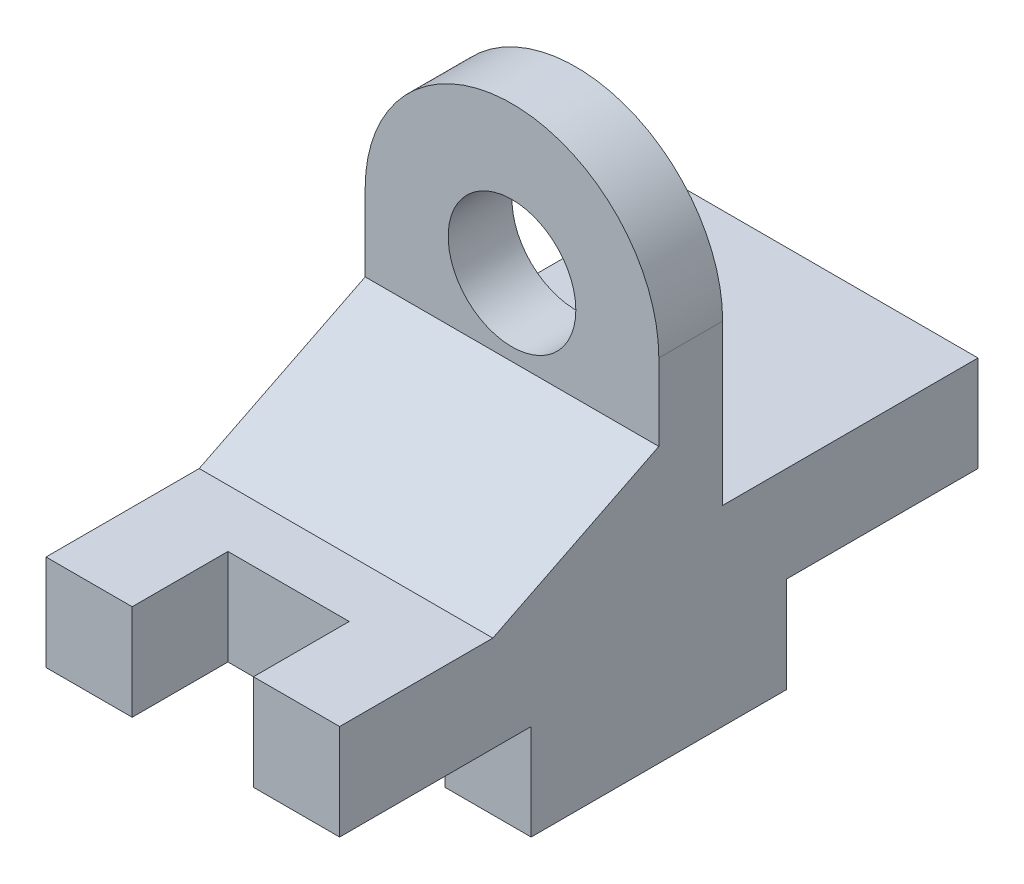
ISO-10303-21;
HEADER;
FILE_DESCRIPTION(('STEP AP214'),'2;1');
FILE_NAME('part.step','',(''),(''),'','','');
FILE_SCHEMA(('AUTOMOTIVE_DESIGN { 1 0 10303 214 1 1 1 1 }'));
ENDSEC;
DATA;
#1=APPLICATION_CONTEXT('core data for automotive mechanical design processes');
#2=APPLICATION_PROTOCOL_DEFINITION('international standard','automotive_design',2000,#1);
#3=PRODUCT_CONTEXT('',#1,'mechanical');
#4=PRODUCT('Part','Part','',(#3));
#5=PRODUCT_RELATED_PRODUCT_CATEGORY('part','',(#4));
#6=PRODUCT_DEFINITION_FORMATION('','',#4);
#7=PRODUCT_DEFINITION_CONTEXT('part definition',#1,'design');
#8=PRODUCT_DEFINITION('design','',#6,#7);
#9=PRODUCT_DEFINITION_SHAPE('','',#8);
#10=(LENGTH_UNIT() NAMED_UNIT(*) SI_UNIT(.MILLI.,.METRE.));
#11=(NAMED_UNIT(*) PLANE_ANGLE_UNIT() SI_UNIT($,.RADIAN.));
#12=(NAMED_UNIT(*) SI_UNIT($,.STERADIAN.) SOLID_ANGLE_UNIT());
#13=UNCERTAINTY_MEASURE_WITH_UNIT(LENGTH_MEASURE(1.E-05),#10,'distance_accuracy_value','');
#14=(GEOMETRIC_REPRESENTATION_CONTEXT(3) GLOBAL_UNCERTAINTY_ASSIGNED_CONTEXT((#13)) GLOBAL_UNIT_ASSIGNED_CONTEXT((#10,
#11,#12)) REPRESENTATION_CONTEXT('',''));
#15=CARTESIAN_POINT('',(0.,0.,0.));
#16=DIRECTION('',(0.,0.,1.));
#17=DIRECTION('',(1.,0.,0.));
#18=AXIS2_PLACEMENT_3D('',#15,#16,#17);
#19=CARTESIAN_POINT('',(23.,0.,60.));
#20=DIRECTION('',(0.,-1.,0.));
#21=DIRECTION('',(0.,0.,-1.));
#22=AXIS2_PLACEMENT_3D('',#19,#20,#21);
#23=PLANE('',#22);
#24=DIRECTION('',(0.,0.,1.));
#25=VECTOR('',#24,1.);
#26=CARTESIAN_POINT('',(23.,0.,60.));
#27=LINE('',#26,#25);
#28=CARTESIAN_POINT('',(23.,0.,35.9999999999999));
#29=VERTEX_POINT('',#28);
#30=CARTESIAN_POINT('',(23.,0.,60.));
#31=VERTEX_POINT('',#30);
#32=EDGE_CURVE('E67',#29,#31,#27,.T.);
#33=ORIENTED_EDGE('',*,*,#32,.F.);
#34=DIRECTION('',(-1.,0.,0.));
#35=VECTOR('',#34,1.);
#36=CARTESIAN_POINT('',(23.,0.,36.));
#37=LINE('',#36,#35);
#38=CARTESIAN_POINT('',(-23.,0.,35.9999999999999));
#39=VERTEX_POINT('',#38);
#40=EDGE_CURVE('E71',#29,#39,#37,.T.);
#41=ORIENTED_EDGE('',*,*,#40,.T.);
#42=DIRECTION('',(0.,0.,1.));
#43=VECTOR('',#42,1.);
#44=CARTESIAN_POINT('',(-23.,0.,60.));
#45=LINE('',#44,#43);
#46=CARTESIAN_POINT('',(-23.,0.,60.));
#47=VERTEX_POINT('',#46);
#48=EDGE_CURVE('E314',#39,#47,#45,.T.);
#49=ORIENTED_EDGE('',*,*,#48,.T.);
#50=DIRECTION('',(-1.,0.,0.));
#51=VECTOR('',#50,1.);
#52=CARTESIAN_POINT('',(23.,0.,60.));
#53=LINE('',#52,#51);
#54=CARTESIAN_POINT('',(-9.5,0.,60.));
#55=VERTEX_POINT('',#54);
#56=EDGE_CURVE('E298',#55,#47,#53,.T.);
#57=ORIENTED_EDGE('',*,*,#56,.F.);
#58=DIRECTION('',(0.,0.,1.));
#59=VECTOR('',#58,1.);
#60=CARTESIAN_POINT('',(-9.5,0.,60.));
#61=LINE('',#60,#59);
#62=CARTESIAN_POINT('',(-9.5,0.,45.));
#63=VERTEX_POINT('',#62);
#64=EDGE_CURVE('E257',#63,#55,#61,.T.);
#65=ORIENTED_EDGE('',*,*,#64,.F.);
#66=DIRECTION('',(-1.,0.,0.));
#67=VECTOR('',#66,1.);
#68=CARTESIAN_POINT('',(-9.5,0.,45.));
#69=LINE('',#68,#67);
#70=CARTESIAN_POINT('',(9.5,0.,45.));
#71=VERTEX_POINT('',#70);
#72=EDGE_CURVE('E266',#71,#63,#69,.T.);
#73=ORIENTED_EDGE('',*,*,#72,.F.);
#74=DIRECTION('',(0.,0.,-1.));
#75=VECTOR('',#74,1.);
#76=CARTESIAN_POINT('',(9.5,0.,60.));
#77=LINE('',#76,#75);
#78=CARTESIAN_POINT('',(9.5,0.,60.));
#79=VERTEX_POINT('',#78);
#80=EDGE_CURVE('E263',#79,#71,#77,.T.);
#81=ORIENTED_EDGE('',*,*,#80,.F.);
#82=EDGE_CURVE('E320',#31,#79,#53,.T.);
#83=ORIENTED_EDGE('',*,*,#82,.F.);
#84=EDGE_LOOP('',(#33,#41,#49,#57,#65,#73,#81,#83));
#85=FACE_BOUND('',#84,.T.);
#86=ADVANCED_FACE('F53',(#85),#23,.F.);
#87=CARTESIAN_POINT('',(23.,-15.,30.));
#88=DIRECTION('',(0.,0.,-1.));
#89=DIRECTION('',(0.,1.,0.));
#90=AXIS2_PLACEMENT_3D('',#87,#88,#89);
#91=PLANE('',#90);
#92=DIRECTION('',(0.,-1.,0.));
#93=VECTOR('',#92,1.);
#94=CARTESIAN_POINT('',(9.5,29.2831796509691,30.));
#95=LINE('',#94,#93);
#96=CARTESIAN_POINT('',(9.5,-15.,30.));
#97=VERTEX_POINT('',#96);
#98=CARTESIAN_POINT('',(9.5,-30.,30.));
#99=VERTEX_POINT('',#98);
#100=EDGE_CURVE('E236',#97,#99,#95,.T.);
#101=ORIENTED_EDGE('',*,*,#100,.T.);
#102=DIRECTION('',(-1.,0.,0.));
#103=VECTOR('',#102,1.);
#104=CARTESIAN_POINT('',(23.,-30.,30.));
#105=LINE('',#104,#103);
#106=CARTESIAN_POINT('',(23.,-30.,30.));
#107=VERTEX_POINT('',#106);
#108=EDGE_CURVE('E333',#107,#99,#105,.T.);
#109=ORIENTED_EDGE('',*,*,#108,.F.);
#110=DIRECTION('',(0.,-1.,0.));
#111=VECTOR('',#110,1.);
#112=CARTESIAN_POINT('',(23.,-15.,30.));
#113=LINE('',#112,#111);
#114=CARTESIAN_POINT('',(23.,-15.,30.));
#115=VERTEX_POINT('',#114);
#116=EDGE_CURVE('E281',#115,#107,#113,.T.);
#117=ORIENTED_EDGE('',*,*,#116,.F.);
#118=DIRECTION('',(-1.,0.,0.));
#119=VECTOR('',#118,1.);
#120=CARTESIAN_POINT('',(23.,-15.,30.));
#121=LINE('',#120,#119);
#122=EDGE_CURVE('E336',#115,#97,#121,.T.);
#123=ORIENTED_EDGE('',*,*,#122,.T.);
#124=EDGE_LOOP('',(#101,#109,#117,#123));
#125=FACE_BOUND('',#124,.T.);
#126=ADVANCED_FACE('F399',(#125),#91,.F.);
#127=CARTESIAN_POINT('',(23.,-30.,30.));
#128=DIRECTION('',(0.,1.,0.));
#129=DIRECTION('',(0.,0.,1.));
#130=AXIS2_PLACEMENT_3D('',#127,#128,#129);
#131=PLANE('',#130);
#132=DIRECTION('',(0.,0.,1.));
#133=VECTOR('',#132,1.);
#134=CARTESIAN_POINT('',(9.5,-30.,30.));
#135=LINE('',#134,#133);
#136=CARTESIAN_POINT('',(9.5,-30.,-10.));
#137=VERTEX_POINT('',#136);
#138=EDGE_CURVE('E232',#99,#137,#135,.F.);
#139=ORIENTED_EDGE('',*,*,#138,.T.);
#140=DIRECTION('',(-1.,0.,0.));
#141=VECTOR('',#140,1.);
#142=CARTESIAN_POINT('',(23.,-30.,-10.));
#143=LINE('',#142,#141);
#144=CARTESIAN_POINT('',(23.,-30.,-10.));
#145=VERTEX_POINT('',#144);
#146=EDGE_CURVE('E332',#145,#137,#143,.T.);
#147=ORIENTED_EDGE('',*,*,#146,.F.);
#148=DIRECTION('',(0.,0.,-1.));
#149=VECTOR('',#148,1.);
#150=CARTESIAN_POINT('',(23.,-30.,30.));
#151=LINE('',#150,#149);
#152=EDGE_CURVE('E282',#107,#145,#151,.T.);
#153=ORIENTED_EDGE('',*,*,#152,.F.);
#154=ORIENTED_EDGE('',*,*,#108,.T.);
#155=EDGE_LOOP('',(#139,#147,#153,#154));
#156=FACE_BOUND('',#155,.T.);
#157=ADVANCED_FACE('F400',(#156),#131,.F.);
#158=CARTESIAN_POINT('',(23.,-30.,-10.));
#159=DIRECTION('',(0.,0.,1.));
#160=DIRECTION('',(1.,0.,0.));
#161=AXIS2_PLACEMENT_3D('',#158,#159,#160);
#162=PLANE('',#161);
#163=DIRECTION('',(0.,-1.,0.));
#164=VECTOR('',#163,1.);
#165=CARTESIAN_POINT('',(9.5,29.2831796509691,-10.));
#166=LINE('',#165,#164);
#167=CARTESIAN_POINT('',(9.5,-15.,-10.));
#168=VERTEX_POINT('',#167);
#169=EDGE_CURVE('E240',#168,#137,#166,.T.);
#170=ORIENTED_EDGE('',*,*,#169,.F.);
#171=DIRECTION('',(-1.,0.,0.));
#172=VECTOR('',#171,1.);
#173=CARTESIAN_POINT('',(23.,-15.,-10.));
#174=LINE('',#173,#172);
#175=CARTESIAN_POINT('',(23.,-15.,-10.));
#176=VERTEX_POINT('',#175);
#177=EDGE_CURVE('E330',#176,#168,#174,.T.);
#178=ORIENTED_EDGE('',*,*,#177,.F.);
#179=DIRECTION('',(0.,1.,0.));
#180=VECTOR('',#179,1.);
#181=CARTESIAN_POINT('',(23.,-30.,-10.));
#182=LINE('',#181,#180);
#183=EDGE_CURVE('E290',#145,#176,#182,.T.);
#184=ORIENTED_EDGE('',*,*,#183,.F.);
#185=ORIENTED_EDGE('',*,*,#146,.T.);
#186=EDGE_LOOP('',(#170,#178,#184,#185));
#187=FACE_BOUND('',#186,.T.);
#188=ADVANCED_FACE('F395',(#187),#162,.F.);
#189=CARTESIAN_POINT('',(23.,0.,60.));
#190=DIRECTION('',(0.,0.,-1.));
#191=DIRECTION('',(-1.,0.,0.));
#192=AXIS2_PLACEMENT_3D('',#189,#190,#191);
#193=PLANE('',#192);
#194=ORIENTED_EDGE('',*,*,#82,.T.);
#195=DIRECTION('',(0.,1.,0.));
#196=VECTOR('',#195,1.);
#197=CARTESIAN_POINT('',(9.5,-30.001,60.));
#198=LINE('',#197,#196);
#199=CARTESIAN_POINT('',(9.5,-15.,60.));
#200=VERTEX_POINT('',#199);
#201=EDGE_CURVE('E274',#200,#79,#198,.T.);
#202=ORIENTED_EDGE('',*,*,#201,.F.);
#203=DIRECTION('',(-1.,0.,0.));
#204=VECTOR('',#203,1.);
#205=CARTESIAN_POINT('',(23.,-15.,60.));
#206=LINE('',#205,#204);
#207=CARTESIAN_POINT('',(23.,-15.,60.));
#208=VERTEX_POINT('',#207);
#209=EDGE_CURVE('E12',#208,#200,#206,.T.);
#210=ORIENTED_EDGE('',*,*,#209,.F.);
#211=DIRECTION('',(0.,-1.,0.));
#212=VECTOR('',#211,1.);
#213=CARTESIAN_POINT('',(23.,0.,60.));
#214=LINE('',#213,#212);
#215=EDGE_CURVE('E279',#31,#208,#214,.T.);
#216=ORIENTED_EDGE('',*,*,#215,.F.);
#217=EDGE_LOOP('',(#194,#202,#210,#216));
#218=FACE_BOUND('',#217,.T.);
#219=ADVANCED_FACE('F410',(#218),#193,.F.);
#220=CARTESIAN_POINT('',(-23.,0.,-40.));
#221=VERTEX_POINT('',#220);
#222=CARTESIAN_POINT('',(-23.,0.,0.));
#223=VERTEX_POINT('',#222);
#224=EDGE_CURVE('E283',#221,#223,#45,.T.);
#225=ORIENTED_EDGE('',*,*,#224,.T.);
#226=DIRECTION('',(1.,0.,0.));
#227=VECTOR('',#226,1.);
#228=CARTESIAN_POINT('',(-23.,0.,0.));
#229=LINE('',#228,#227);
#230=CARTESIAN_POINT('',(23.,0.,0.));
#231=VERTEX_POINT('',#230);
#232=EDGE_CURVE('E223',#223,#231,#229,.T.);
#233=ORIENTED_EDGE('',*,*,#232,.T.);
#234=CARTESIAN_POINT('',(23.,0.,-40.));
#235=VERTEX_POINT('',#234);
#236=EDGE_CURVE('E291',#235,#231,#27,.T.);
#237=ORIENTED_EDGE('',*,*,#236,.F.);
#238=DIRECTION('',(-1.,0.,0.));
#239=VECTOR('',#238,1.);
#240=CARTESIAN_POINT('',(23.,0.,-40.));
#241=LINE('',#240,#239);
#242=EDGE_CURVE('E319',#235,#221,#241,.T.);
#243=ORIENTED_EDGE('',*,*,#242,.T.);
#244=EDGE_LOOP('',(#225,#233,#237,#243));
#245=FACE_BOUND('',#244,.T.);
#246=ADVANCED_FACE('F377',(#245),#23,.F.);
#247=DIRECTION('',(0.,-1.,0.));
#248=VECTOR('',#247,1.);
#249=CARTESIAN_POINT('',(-23.,0.,60.));
#250=LINE('',#249,#248);
#251=CARTESIAN_POINT('',(-23.,-15.,60.));
#252=VERTEX_POINT('',#251);
#253=EDGE_CURVE('E275',#47,#252,#250,.T.);
#254=ORIENTED_EDGE('',*,*,#253,.T.);
#255=CARTESIAN_POINT('',(-9.5,-15.,60.));
#256=VERTEX_POINT('',#255);
#257=EDGE_CURVE('E65',#256,#252,#206,.T.);
#258=ORIENTED_EDGE('',*,*,#257,.F.);
#259=DIRECTION('',(0.,1.,0.));
#260=VECTOR('',#259,1.);
#261=CARTESIAN_POINT('',(-9.5,-30.001,60.));
#262=LINE('',#261,#260);
#263=EDGE_CURVE('E267',#256,#55,#262,.T.);
#264=ORIENTED_EDGE('',*,*,#263,.T.);
#265=ORIENTED_EDGE('',*,*,#56,.T.);
#266=EDGE_LOOP('',(#254,#258,#264,#265));
#267=FACE_BOUND('',#266,.T.);
#268=ADVANCED_FACE('F57',(#267),#193,.F.);
#269=CARTESIAN_POINT('',(-9.5,-30.,30.));
#270=VERTEX_POINT('',#269);
#271=CARTESIAN_POINT('',(-23.,-30.,30.));
#272=VERTEX_POINT('',#271);
#273=EDGE_CURVE('E331',#270,#272,#105,.T.);
#274=ORIENTED_EDGE('',*,*,#273,.F.);
#275=DIRECTION('',(0.,-1.,0.));
#276=VECTOR('',#275,1.);
#277=CARTESIAN_POINT('',(-9.5,29.2831796509691,30.));
#278=LINE('',#277,#276);
#279=CARTESIAN_POINT('',(-9.5,-15.,30.));
#280=VERTEX_POINT('',#279);
#281=EDGE_CURVE('E248',#280,#270,#278,.T.);
#282=ORIENTED_EDGE('',*,*,#281,.F.);
#283=CARTESIAN_POINT('',(-23.,-15.,30.));
#284=VERTEX_POINT('',#283);
#285=EDGE_CURVE('E340',#280,#284,#121,.T.);
#286=ORIENTED_EDGE('',*,*,#285,.T.);
#287=DIRECTION('',(0.,-1.,0.));
#288=VECTOR('',#287,1.);
#289=CARTESIAN_POINT('',(-23.,-15.,30.));
#290=LINE('',#289,#288);
#291=EDGE_CURVE('E303',#284,#272,#290,.T.);
#292=ORIENTED_EDGE('',*,*,#291,.T.);
#293=EDGE_LOOP('',(#274,#282,#286,#292));
#294=FACE_BOUND('',#293,.T.);
#295=ADVANCED_FACE('F346',(#294),#91,.F.);
#296=CARTESIAN_POINT('',(-9.5,-30.,-10.));
#297=VERTEX_POINT('',#296);
#298=CARTESIAN_POINT('',(-23.,-30.,-10.));
#299=VERTEX_POINT('',#298);
#300=EDGE_CURVE('E329',#297,#299,#143,.T.);
#301=ORIENTED_EDGE('',*,*,#300,.F.);
#302=DIRECTION('',(0.,0.,1.));
#303=VECTOR('',#302,1.);
#304=CARTESIAN_POINT('',(-9.5,-30.,30.));
#305=LINE('',#304,#303);
#306=EDGE_CURVE('E239',#270,#297,#305,.F.);
#307=ORIENTED_EDGE('',*,*,#306,.F.);
#308=ORIENTED_EDGE('',*,*,#273,.T.);
#309=DIRECTION('',(0.,0.,-1.));
#310=VECTOR('',#309,1.);
#311=CARTESIAN_POINT('',(-23.,-30.,30.));
#312=LINE('',#311,#310);
#313=EDGE_CURVE('E302',#272,#299,#312,.T.);
#314=ORIENTED_EDGE('',*,*,#313,.T.);
#315=EDGE_LOOP('',(#301,#307,#308,#314));
#316=FACE_BOUND('',#315,.T.);
#317=ADVANCED_FACE('F363',(#316),#131,.F.);
#318=CARTESIAN_POINT('',(-9.5,-15.,-10.));
#319=VERTEX_POINT('',#318);
#320=CARTESIAN_POINT('',(-23.,-15.,-10.));
#321=VERTEX_POINT('',#320);
#322=EDGE_CURVE('E326',#319,#321,#174,.T.);
#323=ORIENTED_EDGE('',*,*,#322,.F.);
#324=DIRECTION('',(0.,-1.,0.));
#325=VECTOR('',#324,1.);
#326=CARTESIAN_POINT('',(-9.5,29.2831796509691,-10.));
#327=LINE('',#326,#325);
#328=EDGE_CURVE('E242',#319,#297,#327,.T.);
#329=ORIENTED_EDGE('',*,*,#328,.T.);
#330=ORIENTED_EDGE('',*,*,#300,.T.);
#331=DIRECTION('',(0.,1.,0.));
#332=VECTOR('',#331,1.);
#333=CARTESIAN_POINT('',(-23.,-30.,-10.));
#334=LINE('',#333,#332);
#335=EDGE_CURVE('E307',#299,#321,#334,.T.);
#336=ORIENTED_EDGE('',*,*,#335,.T.);
#337=EDGE_LOOP('',(#323,#329,#330,#336));
#338=FACE_BOUND('',#337,.T.);
#339=ADVANCED_FACE('F366',(#338),#162,.F.);
#340=CARTESIAN_POINT('',(23.,-15.,-10.));
#341=DIRECTION('',(0.,1.,0.));
#342=DIRECTION('',(0.,0.,1.));
#343=AXIS2_PLACEMENT_3D('',#340,#341,#342);
#344=PLANE('',#343);
#345=DIRECTION('',(0.,0.,-1.));
#346=VECTOR('',#345,1.);
#347=CARTESIAN_POINT('',(-23.,-15.,-10.));
#348=LINE('',#347,#346);
#349=CARTESIAN_POINT('',(-23.,-15.,-40.));
#350=VERTEX_POINT('',#349);
#351=EDGE_CURVE('E309',#321,#350,#348,.T.);
#352=ORIENTED_EDGE('',*,*,#351,.T.);
#353=DIRECTION('',(-1.,0.,0.));
#354=VECTOR('',#353,1.);
#355=CARTESIAN_POINT('',(23.,-15.,-40.));
#356=LINE('',#355,#354);
#357=CARTESIAN_POINT('',(23.,-15.,-40.));
#358=VERTEX_POINT('',#357);
#359=EDGE_CURVE('E323',#358,#350,#356,.T.);
#360=ORIENTED_EDGE('',*,*,#359,.F.);
#361=DIRECTION('',(0.,0.,-1.));
#362=VECTOR('',#361,1.);
#363=CARTESIAN_POINT('',(23.,-15.,-10.));
#364=LINE('',#363,#362);
#365=EDGE_CURVE('E287',#176,#358,#364,.T.);
#366=ORIENTED_EDGE('',*,*,#365,.F.);
#367=ORIENTED_EDGE('',*,*,#177,.T.);
#368=DIRECTION('',(0.,0.,-1.));
#369=VECTOR('',#368,1.);
#370=CARTESIAN_POINT('',(9.5,-15.,30.));
#371=LINE('',#370,#369);
#372=EDGE_CURVE('E243',#97,#168,#371,.T.);
#373=ORIENTED_EDGE('',*,*,#372,.F.);
#374=ORIENTED_EDGE('',*,*,#122,.F.);
#375=DIRECTION('',(0.,0.,-1.));
#376=VECTOR('',#375,1.);
#377=CARTESIAN_POINT('',(23.,-15.,60.));
#378=LINE('',#377,#376);
#379=EDGE_CURVE('E278',#208,#115,#378,.T.);
#380=ORIENTED_EDGE('',*,*,#379,.F.);
#381=ORIENTED_EDGE('',*,*,#209,.T.);
#382=DIRECTION('',(0.,0.,1.));
#383=VECTOR('',#382,1.);
#384=CARTESIAN_POINT('',(9.5,-15.,60.));
#385=LINE('',#384,#383);
#386=CARTESIAN_POINT('',(9.5,-15.,45.));
#387=VERTEX_POINT('',#386);
#388=EDGE_CURVE('E241',#387,#200,#385,.T.);
#389=ORIENTED_EDGE('',*,*,#388,.F.);
#390=DIRECTION('',(1.,0.,0.));
#391=VECTOR('',#390,1.);
#392=CARTESIAN_POINT('',(-9.5,-15.,45.));
#393=LINE('',#392,#391);
#394=CARTESIAN_POINT('',(-9.5,-15.,45.));
#395=VERTEX_POINT('',#394);
#396=EDGE_CURVE('E255',#395,#387,#393,.T.);
#397=ORIENTED_EDGE('',*,*,#396,.F.);
#398=DIRECTION('',(0.,0.,-1.));
#399=VECTOR('',#398,1.);
#400=CARTESIAN_POINT('',(-9.5,-15.,60.));
#401=LINE('',#400,#399);
#402=EDGE_CURVE('E260',#256,#395,#401,.T.);
#403=ORIENTED_EDGE('',*,*,#402,.F.);
#404=ORIENTED_EDGE('',*,*,#257,.T.);
#405=DIRECTION('',(0.,0.,-1.));
#406=VECTOR('',#405,1.);
#407=CARTESIAN_POINT('',(-23.,-15.,60.));
#408=LINE('',#407,#406);
#409=EDGE_CURVE('E296',#252,#284,#408,.T.);
#410=ORIENTED_EDGE('',*,*,#409,.T.);
#411=ORIENTED_EDGE('',*,*,#285,.F.);
#412=DIRECTION('',(0.,0.,-1.));
#413=VECTOR('',#412,1.);
#414=CARTESIAN_POINT('',(-9.5,-15.,30.));
#415=LINE('',#414,#413);
#416=EDGE_CURVE('E235',#280,#319,#415,.T.);
#417=ORIENTED_EDGE('',*,*,#416,.T.);
#418=ORIENTED_EDGE('',*,*,#322,.T.);
#419=EDGE_LOOP('',(#352,#360,#366,#367,#373,#374,#380,#381,#389,#397,#403,#404,#410,#411,#417,#418));
#420=FACE_BOUND('',#419,.T.);
#421=ADVANCED_FACE('F351',(#420),#344,.F.);
#422=CARTESIAN_POINT('',(23.,-15.,-40.));
#423=DIRECTION('',(0.,0.,1.));
#424=DIRECTION('',(0.,-1.,0.));
#425=AXIS2_PLACEMENT_3D('',#422,#423,#424);
#426=PLANE('',#425);
#427=DIRECTION('',(0.,1.,0.));
#428=VECTOR('',#427,1.);
#429=CARTESIAN_POINT('',(-23.,-15.,-40.));
#430=LINE('',#429,#428);
#431=EDGE_CURVE('E315',#350,#221,#430,.T.);
#432=ORIENTED_EDGE('',*,*,#431,.T.);
#433=ORIENTED_EDGE('',*,*,#242,.F.);
#434=DIRECTION('',(0.,1.,0.));
#435=VECTOR('',#434,1.);
#436=CARTESIAN_POINT('',(23.,-15.,-40.));
#437=LINE('',#436,#435);
#438=EDGE_CURVE('E292',#358,#235,#437,.T.);
#439=ORIENTED_EDGE('',*,*,#438,.F.);
#440=ORIENTED_EDGE('',*,*,#359,.T.);
#441=EDGE_LOOP('',(#432,#433,#439,#440));
#442=FACE_BOUND('',#441,.T.);
#443=ADVANCED_FACE('F372',(#442),#426,.F.);
#444=CARTESIAN_POINT('',(23.,0.,0.));
#445=DIRECTION('',(1.,0.,0.));
#446=DIRECTION('',(0.,0.,-1.));
#447=AXIS2_PLACEMENT_3D('',#444,#445,#446);
#448=PLANE('',#447);
#449=DIRECTION('',(0.,-0.447213595499958,0.894427190999916));
#450=VECTOR('',#449,1.);
#451=CARTESIAN_POINT('',(23.,13.,10.));
#452=LINE('',#451,#450);
#453=CARTESIAN_POINT('',(23.,13.,10.));
#454=VERTEX_POINT('',#453);
#455=EDGE_CURVE('E424',#454,#29,#452,.T.);
#456=ORIENTED_EDGE('',*,*,#455,.T.);
#457=ORIENTED_EDGE('',*,*,#32,.T.);
#458=ORIENTED_EDGE('',*,*,#215,.T.);
#459=ORIENTED_EDGE('',*,*,#379,.T.);
#460=ORIENTED_EDGE('',*,*,#116,.T.);
#461=ORIENTED_EDGE('',*,*,#152,.T.);
#462=ORIENTED_EDGE('',*,*,#183,.T.);
#463=ORIENTED_EDGE('',*,*,#365,.T.);
#464=ORIENTED_EDGE('',*,*,#438,.T.);
#465=ORIENTED_EDGE('',*,*,#236,.T.);
#466=DIRECTION('',(0.,-1.,0.));
#467=VECTOR('',#466,1.);
#468=CARTESIAN_POINT('',(23.,25.,0.));
#469=LINE('',#468,#467);
#470=CARTESIAN_POINT('',(23.,25.,0.));
#471=VERTEX_POINT('',#470);
#472=EDGE_CURVE('E224',#471,#231,#469,.T.);
#473=ORIENTED_EDGE('',*,*,#472,.F.);
#474=DIRECTION('',(0.,0.,-1.));
#475=VECTOR('',#474,1.);
#476=CARTESIAN_POINT('',(23.,25.,10.));
#477=LINE('',#476,#475);
#478=CARTESIAN_POINT('',(23.,25.,10.));
#479=VERTEX_POINT('',#478);
#480=EDGE_CURVE('E213',#479,#471,#477,.T.);
#481=ORIENTED_EDGE('',*,*,#480,.F.);
#482=DIRECTION('',(0.,-1.,0.));
#483=VECTOR('',#482,1.);
#484=CARTESIAN_POINT('',(23.,25.,10.));
#485=LINE('',#484,#483);
#486=EDGE_CURVE('E201',#479,#454,#485,.T.);
#487=ORIENTED_EDGE('',*,*,#486,.T.);
#488=EDGE_LOOP('',(#456,#457,#458,#459,#460,#461,#462,#463,#464,#465,#473,#481,#487));
#489=FACE_BOUND('',#488,.T.);
#490=ADVANCED_FACE('F387',(#489),#448,.T.);
#491=CARTESIAN_POINT('',(-23.,0.,0.));
#492=DIRECTION('',(1.,0.,0.));
#493=DIRECTION('',(0.,0.,-1.));
#494=AXIS2_PLACEMENT_3D('',#491,#492,#493);
#495=PLANE('',#494);
#496=ORIENTED_EDGE('',*,*,#48,.F.);
#497=DIRECTION('',(0.,-0.447213595499958,0.894427190999916));
#498=VECTOR('',#497,1.);
#499=CARTESIAN_POINT('',(-23.,13.,10.));
#500=LINE('',#499,#498);
#501=CARTESIAN_POINT('',(-23.,13.,10.));
#502=VERTEX_POINT('',#501);
#503=EDGE_CURVE('E217',#502,#39,#500,.T.);
#504=ORIENTED_EDGE('',*,*,#503,.F.);
#505=DIRECTION('',(0.,-1.,0.));
#506=VECTOR('',#505,1.);
#507=CARTESIAN_POINT('',(-23.,25.,10.));
#508=LINE('',#507,#506);
#509=CARTESIAN_POINT('',(-23.,25.,10.));
#510=VERTEX_POINT('',#509);
#511=EDGE_CURVE('E199',#510,#502,#508,.T.);
#512=ORIENTED_EDGE('',*,*,#511,.F.);
#513=DIRECTION('',(0.,0.,-1.));
#514=VECTOR('',#513,1.);
#515=CARTESIAN_POINT('',(-23.,25.,10.));
#516=LINE('',#515,#514);
#517=CARTESIAN_POINT('',(-23.,25.,0.));
#518=VERTEX_POINT('',#517);
#519=EDGE_CURVE('E202',#510,#518,#516,.T.);
#520=ORIENTED_EDGE('',*,*,#519,.T.);
#521=DIRECTION('',(0.,-1.,0.));
#522=VECTOR('',#521,1.);
#523=CARTESIAN_POINT('',(-23.,25.,0.));
#524=LINE('',#523,#522);
#525=EDGE_CURVE('E229',#518,#223,#524,.T.);
#526=ORIENTED_EDGE('',*,*,#525,.T.);
#527=ORIENTED_EDGE('',*,*,#224,.F.);
#528=ORIENTED_EDGE('',*,*,#431,.F.);
#529=ORIENTED_EDGE('',*,*,#351,.F.);
#530=ORIENTED_EDGE('',*,*,#335,.F.);
#531=ORIENTED_EDGE('',*,*,#313,.F.);
#532=ORIENTED_EDGE('',*,*,#291,.F.);
#533=ORIENTED_EDGE('',*,*,#409,.F.);
#534=ORIENTED_EDGE('',*,*,#253,.F.);
#535=EDGE_LOOP('',(#496,#504,#512,#520,#526,#527,#528,#529,#530,#531,#532,#533,#534));
#536=FACE_BOUND('',#535,.T.);
#537=ADVANCED_FACE('F216',(#536),#495,.F.);
#538=CARTESIAN_POINT('',(-9.5,-30.001,60.));
#539=DIRECTION('',(-1.,0.,0.));
#540=DIRECTION('',(0.,0.,1.));
#541=AXIS2_PLACEMENT_3D('',#538,#539,#540);
#542=PLANE('',#541);
#543=ORIENTED_EDGE('',*,*,#64,.T.);
#544=ORIENTED_EDGE('',*,*,#263,.F.);
#545=ORIENTED_EDGE('',*,*,#402,.T.);
#546=DIRECTION('',(0.,1.,0.));
#547=VECTOR('',#546,1.);
#548=CARTESIAN_POINT('',(-9.5,-30.001,45.));
#549=LINE('',#548,#547);
#550=EDGE_CURVE('E269',#395,#63,#549,.T.);
#551=ORIENTED_EDGE('',*,*,#550,.T.);
#552=EDGE_LOOP('',(#543,#544,#545,#551));
#553=FACE_BOUND('',#552,.T.);
#554=ADVANCED_FACE('F531',(#553),#542,.F.);
#555=CARTESIAN_POINT('',(-9.5,-30.001,45.));
#556=DIRECTION('',(0.,0.,-1.));
#557=DIRECTION('',(0.,1.,0.));
#558=AXIS2_PLACEMENT_3D('',#555,#556,#557);
#559=PLANE('',#558);
#560=ORIENTED_EDGE('',*,*,#72,.T.);
#561=ORIENTED_EDGE('',*,*,#550,.F.);
#562=ORIENTED_EDGE('',*,*,#396,.T.);
#563=DIRECTION('',(0.,1.,0.));
#564=VECTOR('',#563,1.);
#565=CARTESIAN_POINT('',(9.5,-30.001,45.));
#566=LINE('',#565,#564);
#567=EDGE_CURVE('E272',#387,#71,#566,.T.);
#568=ORIENTED_EDGE('',*,*,#567,.T.);
#569=EDGE_LOOP('',(#560,#561,#562,#568));
#570=FACE_BOUND('',#569,.T.);
#571=ADVANCED_FACE('F414',(#570),#559,.F.);
#572=CARTESIAN_POINT('',(9.5,-30.001,60.));
#573=DIRECTION('',(1.,0.,0.));
#574=DIRECTION('',(0.,0.,-1.));
#575=AXIS2_PLACEMENT_3D('',#572,#573,#574);
#576=PLANE('',#575);
#577=ORIENTED_EDGE('',*,*,#80,.T.);
#578=ORIENTED_EDGE('',*,*,#567,.F.);
#579=ORIENTED_EDGE('',*,*,#388,.T.);
#580=ORIENTED_EDGE('',*,*,#201,.T.);
#581=EDGE_LOOP('',(#577,#578,#579,#580));
#582=FACE_BOUND('',#581,.T.);
#583=ADVANCED_FACE('F407',(#582),#576,.F.);
#584=CARTESIAN_POINT('',(-9.5,29.2831796509691,30.));
#585=DIRECTION('',(-1.,0.,0.));
#586=DIRECTION('',(0.,0.,1.));
#587=AXIS2_PLACEMENT_3D('',#584,#585,#586);
#588=PLANE('',#587);
#589=ORIENTED_EDGE('',*,*,#281,.T.);
#590=ORIENTED_EDGE('',*,*,#306,.T.);
#591=ORIENTED_EDGE('',*,*,#328,.F.);
#592=ORIENTED_EDGE('',*,*,#416,.F.);
#593=EDGE_LOOP('',(#589,#590,#591,#592));
#594=FACE_BOUND('',#593,.T.);
#595=ADVANCED_FACE('F364',(#594),#588,.F.);
#596=CARTESIAN_POINT('',(9.5,29.2831796509691,30.));
#597=DIRECTION('',(-1.,0.,0.));
#598=DIRECTION('',(0.,0.,1.));
#599=AXIS2_PLACEMENT_3D('',#596,#597,#598);
#600=PLANE('',#599);
#601=ORIENTED_EDGE('',*,*,#372,.T.);
#602=ORIENTED_EDGE('',*,*,#169,.T.);
#603=ORIENTED_EDGE('',*,*,#138,.F.);
#604=ORIENTED_EDGE('',*,*,#100,.F.);
#605=EDGE_LOOP('',(#601,#602,#603,#604));
#606=FACE_BOUND('',#605,.T.);
#607=ADVANCED_FACE('F392',(#606),#600,.T.);
#608=CARTESIAN_POINT('',(0.,25.,10.));
#609=DIRECTION('',(0.,0.,1.));
#610=DIRECTION('',(1.,0.,0.));
#611=AXIS2_PLACEMENT_3D('',#608,#609,#610);
#612=PLANE('',#611);
#613=DIRECTION('',(-1.,0.,0.));
#614=VECTOR('',#613,1.);
#615=CARTESIAN_POINT('',(0.,13.,10.));
#616=LINE('',#615,#614);
#617=EDGE_CURVE('E421',#454,#502,#616,.T.);
#618=ORIENTED_EDGE('',*,*,#617,.F.);
#619=ORIENTED_EDGE('',*,*,#486,.F.);
#620=CARTESIAN_POINT('',(0.,25.,10.));
#621=DIRECTION('',(0.,0.,1.));
#622=DIRECTION('',(1.,0.,0.));
#623=AXIS2_PLACEMENT_3D('',#620,#621,#622);
#624=CIRCLE('',#623,23.);
#625=EDGE_CURVE('E194',#479,#510,#624,.T.);
#626=ORIENTED_EDGE('',*,*,#625,.T.);
#627=ORIENTED_EDGE('',*,*,#511,.T.);
#628=EDGE_LOOP('',(#618,#619,#626,#627));
#629=FACE_BOUND('',#628,.T.);
#630=CARTESIAN_POINT('',(0.,25.,10.));
#631=DIRECTION('',(0.,0.,1.));
#632=DIRECTION('',(1.,0.,0.));
#633=AXIS2_PLACEMENT_3D('',#630,#631,#632);
#634=CIRCLE('',#633,10.);
#635=CARTESIAN_POINT('',(10.,25.,10.));
#636=VERTEX_POINT('',#635);
#637=EDGE_CURVE('E228',#636,#636,#634,.T.);
#638=ORIENTED_EDGE('',*,*,#637,.F.);
#639=EDGE_LOOP('',(#638));
#640=FACE_BOUND('',#639,.T.);
#641=ADVANCED_FACE('F197',(#629,#640),#612,.T.);
#642=CARTESIAN_POINT('',(0.,25.,0.));
#643=DIRECTION('',(0.,0.,1.));
#644=DIRECTION('',(1.,0.,0.));
#645=AXIS2_PLACEMENT_3D('',#642,#643,#644);
#646=PLANE('',#645);
#647=CARTESIAN_POINT('',(0.,25.,0.));
#648=DIRECTION('',(0.,0.,1.));
#649=DIRECTION('',(1.,0.,0.));
#650=AXIS2_PLACEMENT_3D('',#647,#648,#649);
#651=CIRCLE('',#650,10.);
#652=CARTESIAN_POINT('',(10.,25.,0.));
#653=VERTEX_POINT('',#652);
#654=EDGE_CURVE('E429',#653,#653,#651,.T.);
#655=ORIENTED_EDGE('',*,*,#654,.T.);
#656=EDGE_LOOP('',(#655));
#657=FACE_BOUND('',#656,.T.);
#658=ORIENTED_EDGE('',*,*,#472,.T.);
#659=ORIENTED_EDGE('',*,*,#232,.F.);
#660=ORIENTED_EDGE('',*,*,#525,.F.);
#661=CARTESIAN_POINT('',(0.,25.,0.));
#662=DIRECTION('',(0.,0.,1.));
#663=DIRECTION('',(1.,0.,0.));
#664=AXIS2_PLACEMENT_3D('',#661,#662,#663);
#665=CIRCLE('',#664,23.);
#666=EDGE_CURVE('E209',#471,#518,#665,.T.);
#667=ORIENTED_EDGE('',*,*,#666,.F.);
#668=EDGE_LOOP('',(#658,#659,#660,#667));
#669=FACE_BOUND('',#668,.T.);
#670=ADVANCED_FACE('F385',(#657,#669),#646,.F.);
#671=CARTESIAN_POINT('',(0.,25.,10.));
#672=DIRECTION('',(0.,0.,-1.));
#673=DIRECTION('',(-1.,0.,0.));
#674=AXIS2_PLACEMENT_3D('',#671,#672,#673);
#675=CYLINDRICAL_SURFACE('',#674,23.);
#676=ORIENTED_EDGE('',*,*,#666,.T.);
#677=ORIENTED_EDGE('',*,*,#519,.F.);
#678=ORIENTED_EDGE('',*,*,#625,.F.);
#679=ORIENTED_EDGE('',*,*,#480,.T.);
#680=EDGE_LOOP('',(#676,#677,#678,#679));
#681=FACE_BOUND('',#680,.T.);
#682=ADVANCED_FACE('F208',(#681),#675,.T.);
#683=CARTESIAN_POINT('',(0.,25.,10.));
#684=DIRECTION('',(0.,0.,-1.));
#685=DIRECTION('',(-1.,0.,0.));
#686=AXIS2_PLACEMENT_3D('',#683,#684,#685);
#687=CYLINDRICAL_SURFACE('',#686,10.);
#688=ORIENTED_EDGE('',*,*,#654,.F.);
#689=EDGE_LOOP('',(#688));
#690=FACE_BOUND('',#689,.T.);
#691=ORIENTED_EDGE('',*,*,#637,.T.);
#692=EDGE_LOOP('',(#691));
#693=FACE_BOUND('',#692,.T.);
#694=ADVANCED_FACE('F436',(#690,#693),#687,.F.);
#695=CARTESIAN_POINT('',(0.,13.,10.));
#696=DIRECTION('',(0.,0.894427190999916,0.447213595499958));
#697=DIRECTION('',(0.,-0.447213595499958,0.894427190999916));
#698=AXIS2_PLACEMENT_3D('',#695,#696,#697);
#699=PLANE('',#698);
#700=ORIENTED_EDGE('',*,*,#40,.F.);
#701=ORIENTED_EDGE('',*,*,#455,.F.);
#702=ORIENTED_EDGE('',*,*,#617,.T.);
#703=ORIENTED_EDGE('',*,*,#503,.T.);
#704=EDGE_LOOP('',(#700,#701,#702,#703));
#705=FACE_BOUND('',#704,.T.);
#706=ADVANCED_FACE('F423',(#705),#699,.T.);
#707=CLOSED_SHELL('',(#86,#126,#157,#188,#219,#246,#268,#295,#317,#339,#421,#443,#490,#537,#554,
#571,#583,#595,#607,#641,#670,#682,#694,#706));
#708=MANIFOLD_SOLID_BREP('B2',#707);
#709=ADVANCED_BREP_SHAPE_REPRESENTATION('',(#18,#708),#14);
#710=SHAPE_DEFINITION_REPRESENTATION(#9,#709);
ENDSEC;
END-ISO-10303-21;
